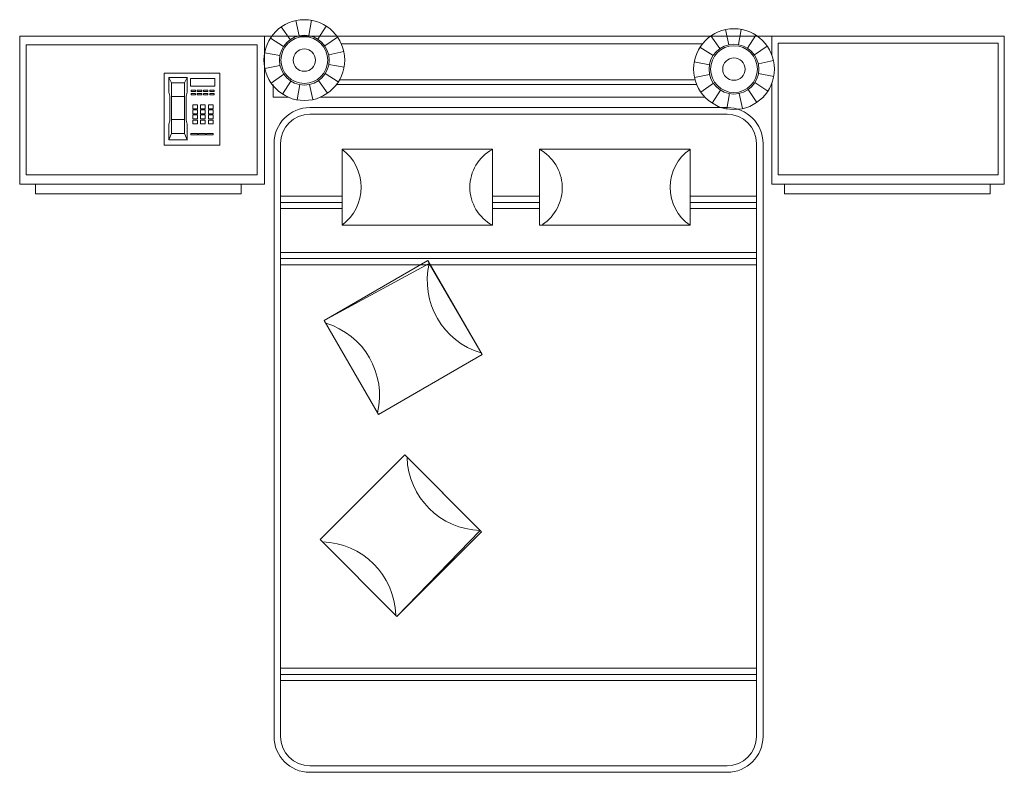
# Model space of a CAD drawing. Units: inches. Extents: x -349 to 9053, y 635 to 6001.
# Tile 7 of 7: x 6173 to 9053, y 3799 to 6001. Entities that reach past the tile are written whole.
import ezdxf

# ---------------------------------------------------------------- set-up
doc = ezdxf.new("R2010")
doc.units = ezdxf.units.IN
doc.layers.add('A-FURN', color=8, linetype='Continuous', lineweight=18)

# ---------------------------------------------------------------- blocks, each defined once
blk = doc.blocks.new('A$C18EB7ED0')
for p, q in [((0.8076, 2.1998), (0.8172, 2.1555)), ((0.8537, 2.2006), (0.8456, 2.1559)), ((0.7653, 2.1814), (0.7911, 2.1442)), ((0.8966, 2.1836), (0.8721, 2.1455)), ((2.0643, 2.1733), (2.0739, 2.129)), ((2.1105, 2.1741), (2.1024, 2.1295)), ((0, 2.1539), (2.8801, 2.1539)), ((0, 1.7209), (0, 2.1539)), ((0.7156, 2.1539), (0.7156, 1.7209)), ((0.7332, 2.1483), (0.7713, 2.1237)), ((0.9298, 2.1515), (0.8925, 2.1257)), ((0.941, 2.1314), (1.9968, 2.1314)), ((2.022, 2.155), (2.0478, 2.1177)), ((2.1534, 2.1571), (2.1288, 2.119)), ((2.1997, 2.1), (2.1997, 2.1539)), ((2.2184, 2.1337), (2.8624, 2.1337)), ((2.2184, 1.7489), (2.2184, 2.1337)), ((2.8624, 2.1337), (2.8624, 1.7489)), ((2.8801, 2.1539), (2.8801, 1.7209)), ((0.0187, 2.129), (0.695, 2.129)), ((0.0187, 1.7489), (0.0187, 2.129)), ((0.695, 2.129), (0.695, 1.7489)), ((0.7162, 2.1054), (0.7608, 2.0973)), ((0.9481, 2.1092), (0.9038, 2.0996)), ((1.9899, 2.1218), (2.028, 2.0973)), ((2.1865, 2.1251), (2.1493, 2.0992)), ((1.973, 2.0789), (2.0176, 2.0708)), ((2.2049, 2.0827), (2.1606, 2.0731)), ((0.5857, 2.0461), (0.4227, 2.0461)), ((0.4227, 2.0461), (0.4227, 1.8353)), ((0.5857, 1.8353), (0.5857, 2.0461)), ((0.717, 2.0593), (0.7613, 2.0688)), ((0.9489, 2.0631), (0.9043, 2.0712)), ((0.4366, 2.0335), (0.4439, 2.018)), ((0.4903, 2.0335), (0.4366, 2.0335)), ((0.4366, 2.0335), (0.4366, 1.9902)), ((0.4824, 2.018), (0.4439, 2.018)), ((0.4824, 2.018), (0.4439, 2.018)), ((0.4439, 2.018), (0.4439, 1.8697)), ((0.4824, 2.018), (0.4903, 2.0335)), ((0.4824, 1.8697), (0.4824, 2.018)), ((0.4903, 1.9902), (0.4903, 2.0338)), ((0.5706, 2.0307), (0.4996, 2.0307)), ((0.4996, 2.0307), (0.4996, 2.0082)), ((0.5706, 2.0082), (0.5706, 2.0307)), ((0.7353, 2.0169), (0.7726, 2.0427)), ((0.7685, 1.9849), (0.7931, 2.023)), ((0.8999, 1.987), (0.8741, 2.0243)), ((0.9319, 2.0202), (0.8938, 2.0447)), ((1.9752, 2.0268), (0.9359, 2.0268)), ((1.9737, 2.0328), (2.0181, 2.0424)), ((1.9921, 1.9905), (2.0294, 2.0163)), ((2.1887, 1.9937), (2.1506, 2.0183)), ((2.2056, 2.0366), (2.161, 2.0447)), ((0.4366, 1.9902), (0.4391, 1.9789)), ((0.4903, 1.9902), (0.4871, 1.9789)), ((0.4996, 2.0082), (0.5706, 2.0082)), ((0.514, 1.9963), (0.5013, 1.9963)), ((0.5013, 1.9963), (0.5013, 1.992)), ((0.5013, 1.992), (0.514, 1.992)), ((0.514, 1.992), (0.514, 1.9963)), ((0.5324, 1.9963), (0.5196, 1.9963)), ((0.5196, 1.9963), (0.5196, 1.992)), ((0.5196, 1.992), (0.5324, 1.992)), ((0.5324, 1.992), (0.5324, 1.9963)), ((0.5507, 1.9963), (0.538, 1.9963)), ((0.538, 1.9963), (0.538, 1.992)), ((0.538, 1.992), (0.5507, 1.992)), ((0.5507, 1.992), (0.5507, 1.9963)), ((0.5691, 1.9963), (0.5564, 1.9963)), ((0.5564, 1.9963), (0.5564, 1.992)), ((0.5564, 1.992), (0.5691, 1.992)), ((0.5691, 1.992), (0.5691, 1.9963)), ((0.7411, 2.0132), (0.7411, 1.9754)), ((0.8114, 1.9679), (0.8195, 2.0125)), ((0.8575, 1.9687), (0.848, 2.013)), ((1.9798, 2.0132), (0.9271, 2.0132)), ((2.0252, 1.9584), (2.0498, 1.9965)), ((2.1566, 1.9605), (2.1308, 1.9978)), ((2.1997, 1.7209), (2.1997, 2.0155)), ((0.4391, 1.9789), (0.4391, 1.9067)), ((0.4824, 1.978), (0.4439, 1.978)), ((0.4871, 1.9789), (0.4871, 1.908)), ((0.514, 1.9864), (0.5013, 1.9864)), ((0.5013, 1.9864), (0.5013, 1.9821)), ((0.5013, 1.9821), (0.514, 1.9821)), ((0.514, 1.9821), (0.514, 1.9864)), ((0.5324, 1.9864), (0.5196, 1.9864)), ((0.5196, 1.9864), (0.5196, 1.9821)), ((0.5196, 1.9821), (0.5324, 1.9821)), ((0.5324, 1.9821), (0.5324, 1.9864)), ((0.5507, 1.9864), (0.538, 1.9864)), ((0.538, 1.9864), (0.538, 1.9821)), ((0.538, 1.9821), (0.5507, 1.9821)), ((0.5507, 1.9821), (0.5507, 1.9864)), ((0.5691, 1.9864), (0.5564, 1.9864)), ((0.5564, 1.9864), (0.5564, 1.9821)), ((0.5564, 1.9821), (0.5691, 1.9821)), ((0.5691, 1.9821), (0.5691, 1.9864)), ((0.7411, 1.9754), (0.7863, 1.9754)), ((0.8788, 1.9754), (2.0045, 1.9754)), ((2.0682, 1.9414), (2.0763, 1.986)), ((2.1143, 1.9422), (2.1047, 1.9865)), ((2.1742, 1.9754), (2.1771, 1.9754)), ((2.1771, 1.9754), (2.1771, 1.9785)), ((0.52, 1.9534), (0.5062, 1.9534)), ((0.5062, 1.9534), (0.5062, 1.9417)), ((0.5062, 1.9417), (0.52, 1.9417)), ((0.52, 1.9385), (0.5062, 1.9385)), ((0.5062, 1.9385), (0.5062, 1.9269)), ((0.52, 1.9417), (0.52, 1.9534)), ((0.52, 1.9269), (0.52, 1.9385)), ((0.5426, 1.9534), (0.5288, 1.9534)), ((0.5288, 1.9534), (0.5288, 1.9417)), ((0.5288, 1.9417), (0.5426, 1.9417)), ((0.5426, 1.9385), (0.5288, 1.9385)), ((0.5288, 1.9385), (0.5288, 1.9269)), ((0.5426, 1.9417), (0.5426, 1.9534)), ((0.5426, 1.9269), (0.5426, 1.9385)), ((0.5659, 1.9534), (0.5521, 1.9534)), ((0.5521, 1.9534), (0.5521, 1.9417)), ((0.5521, 1.9417), (0.5659, 1.9417)), ((0.5659, 1.9385), (0.5521, 1.9385)), ((0.5521, 1.9385), (0.5521, 1.9269)), ((0.5659, 1.9417), (0.5659, 1.9534)), ((0.5659, 1.9269), (0.5659, 1.9385)), ((2.0691, 1.9452), (0.8491, 1.9452)), ((0.4391, 1.9067), (0.4366, 1.8971)), ((0.4439, 1.9101), (0.4824, 1.9101)), ((0.4871, 1.908), (0.4903, 1.8971)), ((0.5062, 1.9269), (0.52, 1.9269)), ((0.52, 1.9237), (0.5062, 1.9237)), ((0.5062, 1.9237), (0.5062, 1.9121)), ((0.5062, 1.9121), (0.52, 1.9121)), ((0.52, 1.9089), (0.5062, 1.9089)), ((0.5062, 1.9089), (0.5062, 1.8972)), ((0.52, 1.9121), (0.52, 1.9237)), ((0.52, 1.8972), (0.52, 1.9089)), ((0.5288, 1.9269), (0.5426, 1.9269)), ((0.5426, 1.9237), (0.5288, 1.9237)), ((0.5288, 1.9237), (0.5288, 1.9121)), ((0.5288, 1.9121), (0.5426, 1.9121)), ((0.5426, 1.9089), (0.5288, 1.9089)), ((0.5288, 1.9089), (0.5288, 1.8972)), ((0.5426, 1.9121), (0.5426, 1.9237)), ((0.5426, 1.8972), (0.5426, 1.9089)), ((0.5521, 1.9269), (0.5659, 1.9269)), ((0.5659, 1.9237), (0.5521, 1.9237)), ((0.5521, 1.9237), (0.5521, 1.9121)), ((0.5521, 1.9121), (0.5659, 1.9121)), ((0.5659, 1.9089), (0.5521, 1.9089)), ((0.5521, 1.9089), (0.5521, 1.8972)), ((0.5659, 1.9121), (0.5659, 1.9237)), ((0.5659, 1.8972), (0.5659, 1.9089)), ((2.0691, 1.926), (0.8491, 1.926)), ((0.4366, 1.8971), (0.4366, 1.8504)), ((0.4903, 1.8499), (0.4903, 1.8971)), ((0.5062, 1.8972), (0.52, 1.8972)), ((0.5288, 1.8972), (0.5426, 1.8972)), ((0.5521, 1.8972), (0.5659, 1.8972)), ((0.4439, 1.8697), (0.4366, 1.8504)), ((0.4366, 1.8504), (0.4903, 1.8504)), ((0.4824, 1.8697), (0.4439, 1.8697)), ((0.4439, 1.8697), (0.4824, 1.8697)), ((0.4903, 1.8504), (0.4824, 1.8697)), ((0.5208, 1.8697), (0.5009, 1.8697)), ((0.5009, 1.8697), (0.5009, 1.8657)), ((0.5009, 1.8657), (0.5208, 1.8657)), ((0.5208, 1.8657), (0.5208, 1.8697)), ((0.5433, 1.8697), (0.5234, 1.8697)), ((0.5234, 1.8697), (0.5234, 1.8657)), ((0.5234, 1.8657), (0.5433, 1.8657)), ((0.5433, 1.8657), (0.5433, 1.8697)), ((0.5658, 1.8697), (0.546, 1.8697)), ((0.546, 1.8697), (0.546, 1.8657)), ((0.546, 1.8657), (0.5658, 1.8657)), ((0.5658, 1.8657), (0.5658, 1.8697)), ((0.4227, 1.8353), (0.5857, 1.8353)), ((0.7439, 1.8401), (0.7439, 0.1052)), ((0.7632, 1.8401), (0.7632, 0.1052)), ((0.9429, 1.8231), (1.3829, 1.8231)), ((0.9429, 1.601), (0.9429, 1.8231)), ((1.3829, 1.8231), (1.3829, 1.601)), ((1.5207, 1.601), (1.5207, 1.8231)), ((1.5207, 1.8231), (1.9608, 1.8231)), ((1.9608, 1.8231), (1.9608, 1.601)), ((2.155, 0.1052), (2.155, 1.8401)), ((2.1743, 0.1052), (2.1743, 1.8401)), ((0.695, 1.7489), (0.0187, 1.7489)), ((2.8624, 1.7489), (2.2184, 1.7489)), ((0.7156, 1.7209), (0, 1.7209)), ((0, 1.7209), (0.6483, 1.7209)), ((0.0462, 1.6929), (0.0462, 1.7209)), ((0.6483, 1.7209), (0.6483, 1.6929)), ((2.8801, 1.7209), (2.1997, 1.7209)), ((2.2369, 1.7209), (2.8801, 1.7209)), ((2.2369, 1.6929), (2.2369, 1.7209)), ((2.839, 1.7209), (2.839, 1.6929)), ((0.6483, 1.6929), (0.0462, 1.6929)), ((0.7632, 1.6858), (0.9429, 1.6858)), ((1.3829, 1.6858), (1.5207, 1.6858)), ((1.9608, 1.6858), (2.155, 1.6858)), ((2.839, 1.6929), (2.2369, 1.6929)), ((0.7632, 1.6678), (0.9429, 1.6678)), ((0.7632, 1.6498), (0.9429, 1.6498)), ((1.3829, 1.6678), (1.5207, 1.6678)), ((1.3829, 1.6498), (1.5207, 1.6498)), ((1.9608, 1.6678), (2.155, 1.6678)), ((1.9608, 1.6498), (2.155, 1.6498)), ((1.3829, 1.601), (0.9429, 1.601)), ((1.9608, 1.601), (1.5207, 1.601)), ((0.7632, 1.5215), (2.155, 1.5215)), ((0.7632, 1.5035), (2.155, 1.5035)), ((0.7632, 1.4855), (2.155, 1.4855)), ((0.8904, 1.3226), (1.1935, 1.4976)), ((0.8904, 1.3226), (1.1982, 1.4894)), ((1.1935, 1.4976), (1.3524, 1.2224)), ((1.1982, 1.4894), (1.3524, 1.2224)), ((1.0493, 1.0474), (0.8904, 1.3226)), ((1.0493, 1.0474), (0.8904, 1.3226)), ((1.3524, 1.2224), (1.0493, 1.0474)), ((1.3524, 1.2224), (1.0493, 1.0474)), ((0.8789, 0.6811), (1.1264, 0.9286)), ((0.8789, 0.6811), (1.1264, 0.9286)), ((1.1264, 0.9286), (1.3473, 0.7077)), ((1.1264, 0.9286), (1.3511, 0.7039)), ((1.3473, 0.7077), (1.1036, 0.4564)), ((1.3511, 0.7039), (1.1036, 0.4564)), ((1.1036, 0.4564), (0.8789, 0.6811)), ((1.1036, 0.4564), (0.8789, 0.6811)), ((0.7632, 0.3045), (2.155, 0.3045)), ((0.7632, 0.2865), (2.155, 0.2865)), ((0.7632, 0.2685), (2.155, 0.2685)), ((0.8491, 0.0193), (2.0691, 0.0193)), ((0.8491, 0), (2.0691, 0))]:
    blk.add_line(p, q)
for centre, radius in [((0.8326, 2.0842), 0.1182), ((2.0893, 2.0578), 0.1182), ((0.8326, 2.0842), 0.0729), ((0.8326, 2.0842), 0.0684), ((0.8326, 2.0842), 0.0328), ((2.0893, 2.0578), 0.0729), ((2.0893, 2.0578), 0.0684), ((2.0893, 2.0578), 0.0328)]:
    blk.add_circle(centre, radius)
for centre, radius, start, end in [((0.8491, 1.8401), 0.1052, 90, 180), ((2.0691, 1.8401), 0.1052, 0, 90), ((0.8491, 1.8401), 0.0859, 90, 180), ((2.0691, 1.8401), 0.0859, 0, 90), ((0.8604, 1.712), 0.1383, 306.5959, 53.4041), ((1.4431, 1.712), 0.1263, 118.4619, 241.5381), ((1.4584, 1.7106), 0.1286, 303.4023, 61.0264), ((2.0371, 1.712), 0.1347, 124.5027, 235.4973), ((1.4126, 1.4383), 0.2204, 166.5879, 253.4121), ((0.8322, 1.1031), 0.2204, 346.5879, 73.4121), ((1.3534, 0.928), 0.2204, 181.5879, 268.4121), ((0.8795, 0.4541), 0.2204, 1.5879, 88.4121), ((0.8491, 0.1052), 0.1052, 180, 270), ((0.8491, 0.1052), 0.0859, 180, 270), ((2.0691, 0.1052), 0.1052, 270, 0), ((2.0691, 0.1052), 0.0859, 270, 0)]:
    blk.add_arc(centre, radius, start, end)

msp = doc.modelspace()

# ---------------------------------------------------------------- block references
at = {"layer": 'A-FURN', "xscale": 1000, "yscale": 1000, "zscale": 1000}
msp.add_blockref('A$C18EB7ED0', (6172.947, 3798.5875), dxfattribs=at)

doc.saveas('drawing.dxf')
